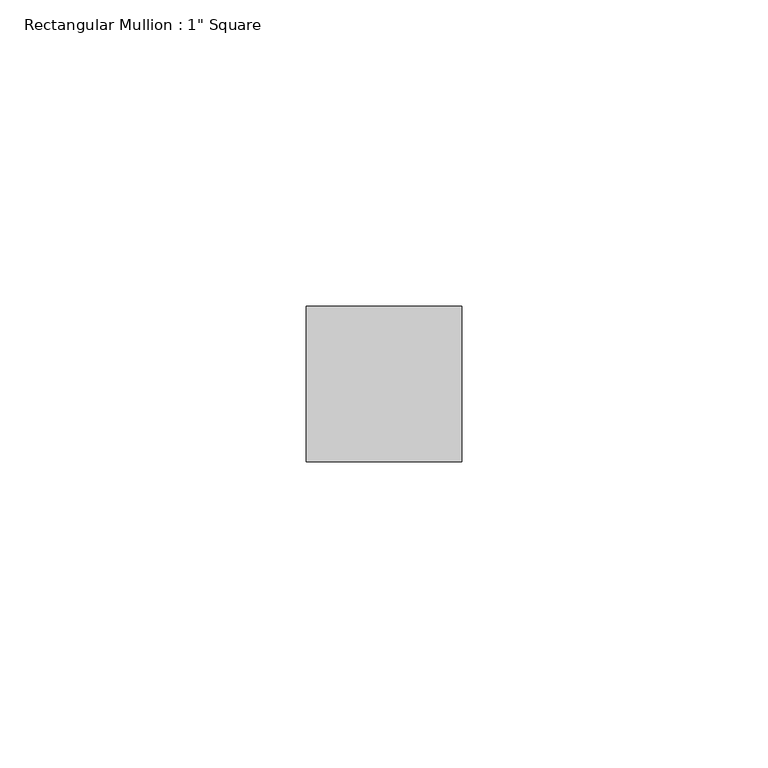
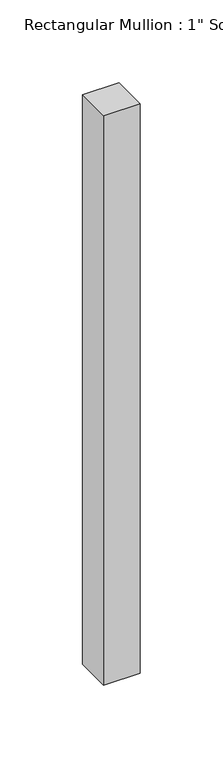
"""IFC4 building model written with IfcOpenShell, lengths in millimetres: member geometry."""

from ifc_helpers import new_model, si_unit, frame, origin, place, context, project, spatial, polyline, outline, extrude, source, transform, mapped, element, save


def member_5dd0e0a2(model_context):
    return source(origin(), model_context, "Body", "SweptSolid", [
        extrude(outline(polyline([(0.0, 12.7), (0.0, -12.7), (-25.4, -12.7), (-25.4, 12.7), (0.0, 12.7)])), frame((0.0, 0.0, -419.1), z_axis=(0.0, 0.0, 1.0), x_axis=(1.0, 0.0, 0.0)), (0.0, 0.0, 1.0), 419.1),
    ])


if __name__ == "__main__":
    model = new_model("IFC4")
    model_context = context("Model", 3, world=origin())
    ifc_project = project(units=[si_unit("LENGTHUNIT", "METRE", prefix="MILLI")], contexts=[model_context])
    site = spatial("IfcSite", under=ifc_project)
    building = spatial("IfcBuilding", under=site)
    placement = place(None, origin())
    member_shape = member_5dd0e0a2(model_context)
    element("IfcMember", 1, ObjectType="Rectangular Mullion : 1\" Square", at=placement, inside=building, context=model_context, shape_type="MappedRepresentation", body=[
        mapped(member_shape, transform((0.0, 0.0, 0.0), x_axis=(1.0, 0.0, 0.0), y_axis=(0.0, 1.0, 0.0), z_axis=(0.0, 0.0, 1.0))),
    ])
    save(model, "model.ifc")

# Revit data of these elements
# Type "Rectangular Mullion : 1\" Square"
#   built-in parameter 1007304 = 0.0833333 (stored number, unit not read)
#   built-in parameter 1007301 = 0.0416667 (stored number, unit not read)
#   built-in parameter 1007300 = 0.0416667 (stored number, unit not read)
